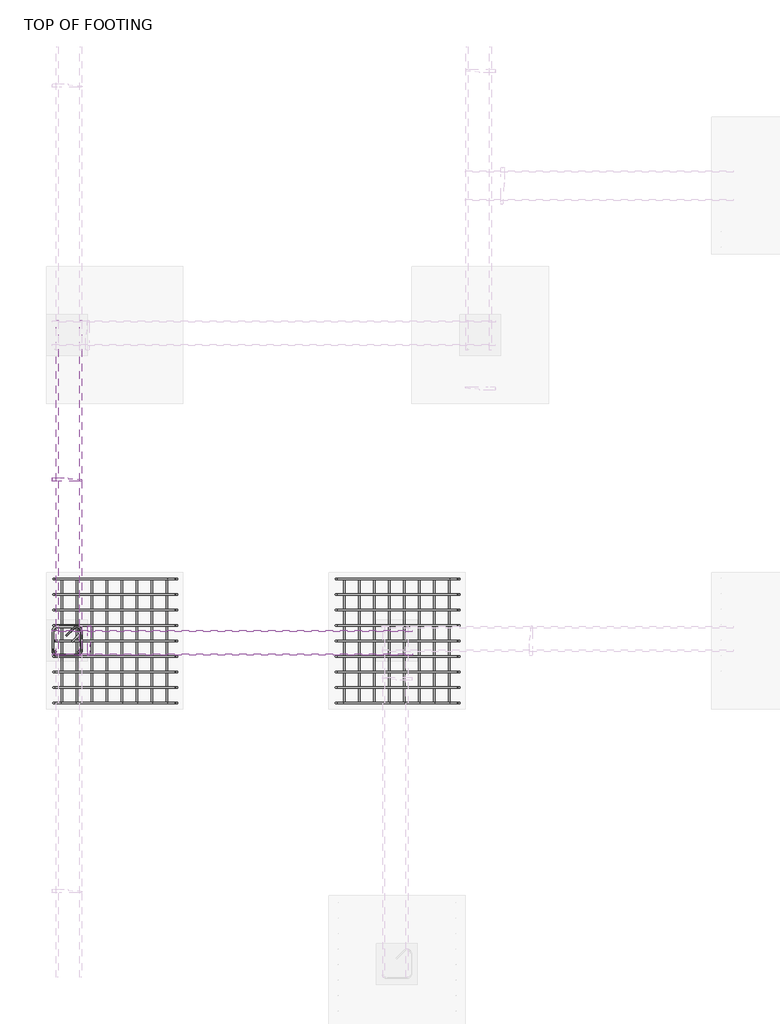
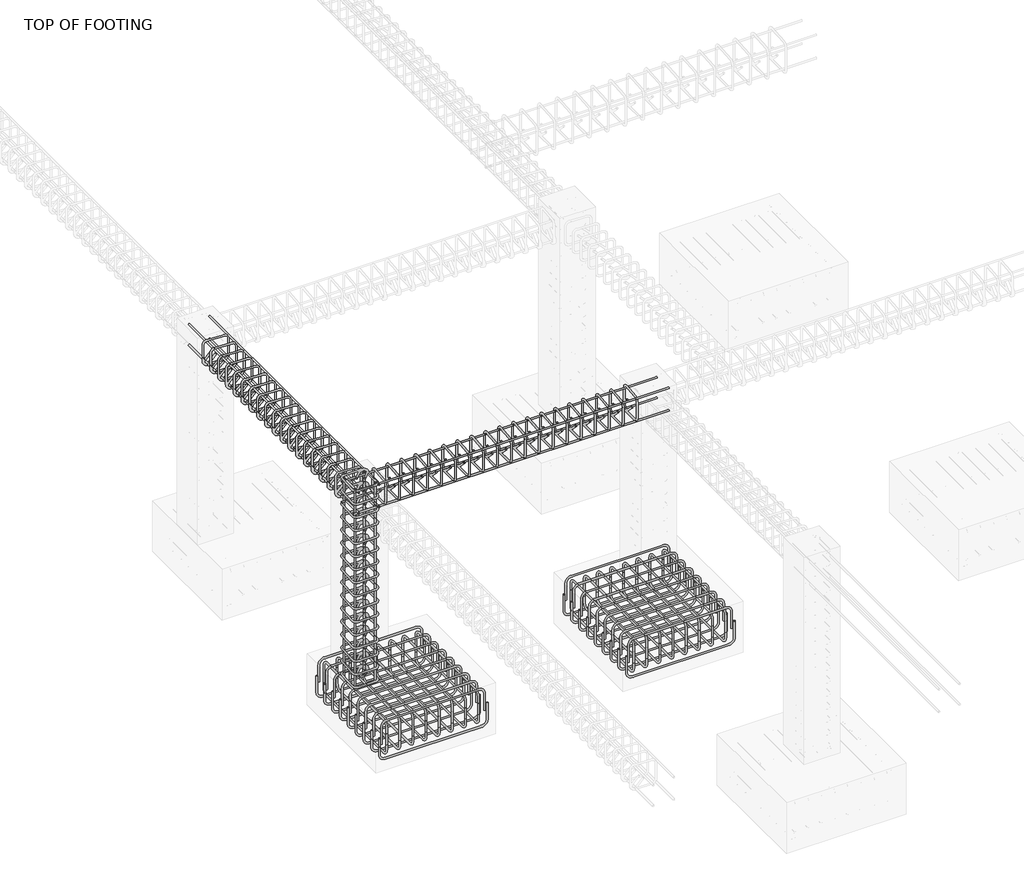
# One storey, part 4 of 10: 17 reinforcing bars.
"""IFC4 building model written with IfcOpenShell, lengths in millimetres."""

from ifc_helpers import new_model, si_unit, point, frame, origin, place, context, project, spatial, polyline, circle_curve, trimmed, segment, composite_curve, source, transform, mapped, element, save
from ifc_brep_helpers import swept_disk

model = new_model("IFC4")

# Units and contexts
model_context = context("Model", 3, world=origin())
ifc_project = project(units=[si_unit("LENGTHUNIT", "METRE", prefix="MILLI")], contexts=[model_context])

# Site, building, storey
site = spatial("IfcSite", under=ifc_project)
building = spatial("IfcBuilding", under=site)
storey = spatial("IfcBuildingStorey", under=building, Name="TOP OF FOOTING", Elevation=-1828.8)

# Reinforcing bars
placement = place(None, origin())
reinforcing_bar_shape = source(origin(), model_context, "Body", "SolidModel", [
    swept_disk(composite_curve([segment(polyline([(-9737.3957678, 12780.6767485, -2013.6880036), (-9737.3957678, 12780.6767485, -2160.9880036)]), True, "CONTINUOUS"), segment(trimmed(circle_curve(frame((-9783.7457678, 12780.6767485, -2160.9880036), z_axis=(0.0, 1.0, 0.0), x_axis=(46.349999999998545, 0.0, 0.0)), 46.35), [point((-9737.3957678, 12780.6767485, -2160.9880036))], [point((-9783.7457678, 12780.6767485, -2207.3380036))], True, "CARTESIAN"), True, "CONTINUOUS"), segment(polyline([(-9783.7457678, 12780.6767485, -2207.3380036), (-10591.4530437, 12780.6767485, -2207.3380036)]), True, "CONTINUOUS"), segment(trimmed(circle_curve(frame((-10591.4530437, 12780.6767485, -2160.9880036), z_axis=(0.0, 1.0, 0.0), x_axis=(0.0, 0.0, -46.34999999999991)), 46.35), [point((-10591.4530437, 12780.6767485, -2207.3380036))], [point((-10637.8030437, 12780.6767485, -2160.9880036))], True, "CARTESIAN"), True, "CONTINUOUS"), segment(polyline([(-10637.8030437, 12780.6767485, -2160.9880036), (-10637.8030437, 12780.6767485, -2013.6880036)]), True, "CONTINUOUS")], self_intersect=False), 6.35),
])
element("IfcReinforcingBar", 1, at=placement, inside=storey, context=model_context, shape_type="MappedRepresentation", body=[
    mapped(reinforcing_bar_shape, transform((0.0, 0.0, 0.0), x_axis=(1.0, 0.0, 0.0), y_axis=(0.0, 1.0, 0.0), z_axis=(0.0, 0.0, 1.0))),
    mapped(reinforcing_bar_shape, transform((0.0, -113.4125, 0.0), x_axis=(1.0, 0.0, 0.0), y_axis=(0.0, 1.0, 0.0), z_axis=(0.0, 0.0, 1.0))),
    mapped(reinforcing_bar_shape, transform((0.0, -226.825, 0.0), x_axis=(1.0, 0.0, 0.0), y_axis=(0.0, 1.0, 0.0), z_axis=(0.0, 0.0, 1.0))),
    mapped(reinforcing_bar_shape, transform((0.0, -340.2375, 0.0), x_axis=(1.0, 0.0, 0.0), y_axis=(0.0, 1.0, 0.0), z_axis=(0.0, 0.0, 1.0))),
    mapped(reinforcing_bar_shape, transform((0.0, -453.65, 0.0), x_axis=(1.0, 0.0, 0.0), y_axis=(0.0, 1.0, 0.0), z_axis=(0.0, 0.0, 1.0))),
    mapped(reinforcing_bar_shape, transform((0.0, -567.0625, 0.0), x_axis=(1.0, 0.0, 0.0), y_axis=(0.0, 1.0, 0.0), z_axis=(0.0, 0.0, 1.0))),
    mapped(reinforcing_bar_shape, transform((0.0, -680.475, 0.0), x_axis=(1.0, 0.0, 0.0), y_axis=(0.0, 1.0, 0.0), z_axis=(0.0, 0.0, 1.0))),
    mapped(reinforcing_bar_shape, transform((0.0, -793.8875, 0.0), x_axis=(1.0, 0.0, 0.0), y_axis=(0.0, 1.0, 0.0), z_axis=(0.0, 0.0, 1.0))),
    mapped(reinforcing_bar_shape, transform((0.0, -907.3, 0.0), x_axis=(1.0, 0.0, 0.0), y_axis=(0.0, 1.0, 0.0), z_axis=(0.0, 0.0, 1.0))),
])
reinforcing_bar_2_shape = source(origin(), model_context, "Body", "SolidModel", [
    swept_disk(composite_curve([segment(polyline([(-10621.5548549, 12780.6767485, -2068.7560969), (-10621.5548549, 12780.6767485, -1921.4560969)]), True, "CONTINUOUS"), segment(trimmed(circle_curve(frame((-10575.2048549, 12780.6767485, -1921.4560969), z_axis=(0.0, 1.0, 0.0), x_axis=(-46.350000000000364, 0.0, 0.0)), 46.35), [point((-10621.5548549, 12780.6767485, -1921.4560969))], [point((-10575.2048549, 12780.6767485, -1875.1060969))], True, "CARTESIAN"), True, "CONTINUOUS"), segment(polyline([(-10575.2048549, 12780.6767485, -1875.1060969), (-9806.8133686, 12780.6767485, -1875.1060969)]), True, "CONTINUOUS"), segment(trimmed(circle_curve(frame((-9806.8133686, 12780.6767485, -1921.4560969), z_axis=(0.0, 1.0, 0.0), x_axis=(0.0, 0.0, 46.34999999999991)), 46.35), [point((-9806.8133686, 12780.6767485, -1875.1060969))], [point((-9760.4633686, 12780.6767485, -1921.4560969))], True, "CARTESIAN"), True, "CONTINUOUS"), segment(polyline([(-9760.4633686, 12780.6767485, -1921.4560969), (-9760.4633686, 12780.6767485, -2068.7560969)]), True, "CONTINUOUS")], self_intersect=False), 6.35),
])
element("IfcReinforcingBar", 2, at=placement, inside=storey, context=model_context, shape_type="MappedRepresentation", body=[
    mapped(reinforcing_bar_2_shape, transform((0.0, 0.0, 0.0), x_axis=(1.0, 0.0, 0.0), y_axis=(0.0, 1.0, 0.0), z_axis=(0.0, 0.0, 1.0))),
    mapped(reinforcing_bar_2_shape, transform((0.0, -113.4125, 0.0), x_axis=(1.0, 0.0, 0.0), y_axis=(0.0, 1.0, 0.0), z_axis=(0.0, 0.0, 1.0))),
    mapped(reinforcing_bar_2_shape, transform((0.0, -226.825, 0.0), x_axis=(1.0, 0.0, 0.0), y_axis=(0.0, 1.0, 0.0), z_axis=(0.0, 0.0, 1.0))),
    mapped(reinforcing_bar_2_shape, transform((0.0, -340.2375, 0.0), x_axis=(1.0, 0.0, 0.0), y_axis=(0.0, 1.0, 0.0), z_axis=(0.0, 0.0, 1.0))),
    mapped(reinforcing_bar_2_shape, transform((0.0, -453.65, 0.0), x_axis=(1.0, 0.0, 0.0), y_axis=(0.0, 1.0, 0.0), z_axis=(0.0, 0.0, 1.0))),
    mapped(reinforcing_bar_2_shape, transform((0.0, -567.0625, 0.0), x_axis=(1.0, 0.0, 0.0), y_axis=(0.0, 1.0, 0.0), z_axis=(0.0, 0.0, 1.0))),
    mapped(reinforcing_bar_2_shape, transform((0.0, -680.475, 0.0), x_axis=(1.0, 0.0, 0.0), y_axis=(0.0, 1.0, 0.0), z_axis=(0.0, 0.0, 1.0))),
    mapped(reinforcing_bar_2_shape, transform((0.0, -793.8875, 0.0), x_axis=(1.0, 0.0, 0.0), y_axis=(0.0, 1.0, 0.0), z_axis=(0.0, 0.0, 1.0))),
    mapped(reinforcing_bar_2_shape, transform((0.0, -907.3, 0.0), x_axis=(1.0, 0.0, 0.0), y_axis=(0.0, 1.0, 0.0), z_axis=(0.0, 0.0, 1.0))),
])
reinforcing_bar_3_shape = source(origin(), model_context, "Body", "SolidModel", [
    swept_disk(composite_curve([segment(polyline([(-9809.6682872, 12780.6767485, -2087.4821199), (-9809.6682872, 12780.6767485, -1940.1821199)]), True, "CONTINUOUS"), segment(trimmed(circle_curve(frame((-9809.6682872, 12734.3267485, -1940.1821199), z_axis=(1.0, 0.0, 0.0), x_axis=(0.0, 46.350000000000364, 0.0)), 46.35), [point((-9809.6682872, 12780.6767485, -1940.1821199))], [point((-9809.6682872, 12734.3267485, -1893.8321199))], True, "CARTESIAN"), True, "CONTINUOUS"), segment(polyline([(-9809.6682872, 12734.3267485, -1893.8321199), (-9809.6682872, 11919.7267485, -1893.8321199)]), True, "CONTINUOUS"), segment(trimmed(circle_curve(frame((-9809.6682872, 11919.7267485, -1940.1821199), z_axis=(1.0, 0.0, 0.0), x_axis=(0.0, 0.0, 46.350000000000136)), 46.35), [point((-9809.6682872, 11919.7267485, -1893.8321199))], [point((-9809.6682872, 11873.3767485, -1940.1821199))], True, "CARTESIAN"), True, "CONTINUOUS"), segment(polyline([(-9809.6682872, 11873.3767485, -1940.1821199), (-9809.6682872, 11873.3767485, -2087.4821199)]), True, "CONTINUOUS")], self_intersect=False), 6.35),
])
element("IfcReinforcingBar", 3, at=placement, inside=storey, context=model_context, shape_type="MappedRepresentation", body=[
    mapped(reinforcing_bar_3_shape, transform((0.0, 0.0, 0.0), x_axis=(1.0, 0.0, 0.0), y_axis=(0.0, 1.0, 0.0), z_axis=(0.0, 0.0, 1.0))),
    mapped(reinforcing_bar_3_shape, transform((-109.824938, 0.0, 0.0), x_axis=(1.0, 0.0, 0.0), y_axis=(0.0, 1.0, 0.0), z_axis=(0.0, 0.0, 1.0))),
    mapped(reinforcing_bar_3_shape, transform((-219.649876, 0.0, 0.0), x_axis=(1.0, 0.0, 0.0), y_axis=(0.0, 1.0, 0.0), z_axis=(0.0, 0.0, 1.0))),
    mapped(reinforcing_bar_3_shape, transform((-329.474814, 0.0, 0.0), x_axis=(1.0, 0.0, 0.0), y_axis=(0.0, 1.0, 0.0), z_axis=(0.0, 0.0, 1.0))),
    mapped(reinforcing_bar_3_shape, transform((-439.299752, 0.0, 0.0), x_axis=(1.0, 0.0, 0.0), y_axis=(0.0, 1.0, 0.0), z_axis=(0.0, 0.0, 1.0))),
    mapped(reinforcing_bar_3_shape, transform((-549.12469, 0.0, 0.0), x_axis=(1.0, 0.0, 0.0), y_axis=(0.0, 1.0, 0.0), z_axis=(0.0, 0.0, 1.0))),
    mapped(reinforcing_bar_3_shape, transform((-658.949628, 0.0, 0.0), x_axis=(1.0, 0.0, 0.0), y_axis=(0.0, 1.0, 0.0), z_axis=(0.0, 0.0, 1.0))),
    mapped(reinforcing_bar_3_shape, transform((-768.774566, 0.0, 0.0), x_axis=(1.0, 0.0, 0.0), y_axis=(0.0, 1.0, 0.0), z_axis=(0.0, 0.0, 1.0))),
])
reinforcing_bar_4_shape = source(origin(), model_context, "Body", "SolidModel", [
    swept_disk(composite_curve([segment(polyline([(-10578.4428532, 12780.6767485, -1990.1985611), (-10578.4428532, 12780.6767485, -2137.4985611)]), True, "CONTINUOUS"), segment(trimmed(circle_curve(frame((-10578.4428532, 12734.3267485, -2137.4985611), z_axis=(-1.0, 0.0, 0.0), x_axis=(0.0, 46.350000000000364, 0.0)), 46.35), [point((-10578.4428532, 12780.6767485, -2137.4985611))], [point((-10578.4428532, 12734.3267485, -2183.8485611))], True, "CARTESIAN"), True, "CONTINUOUS"), segment(polyline([(-10578.4428532, 12734.3267485, -2183.8485611), (-10578.4428532, 11919.7267485, -2183.8485611)]), True, "CONTINUOUS"), segment(trimmed(circle_curve(frame((-10578.4428532, 11919.7267485, -2137.4985611), z_axis=(-1.0, 0.0, 0.0), x_axis=(0.0, 0.0, -46.34999999999991)), 46.35), [point((-10578.4428532, 11919.7267485, -2183.8485611))], [point((-10578.4428532, 11873.3767485, -2137.4985611))], True, "CARTESIAN"), True, "CONTINUOUS"), segment(polyline([(-10578.4428532, 11873.3767485, -2137.4985611), (-10578.4428532, 11873.3767485, -1990.1985611)]), True, "CONTINUOUS")], self_intersect=False), 6.35),
])
element("IfcReinforcingBar", 4, at=placement, inside=storey, context=model_context, shape_type="MappedRepresentation", body=[
    mapped(reinforcing_bar_4_shape, transform((0.0, 0.0, 0.0), x_axis=(1.0, 0.0, 0.0), y_axis=(0.0, 1.0, 0.0), z_axis=(0.0, 0.0, 1.0))),
    mapped(reinforcing_bar_4_shape, transform((109.824938, 0.0, 0.0), x_axis=(1.0, 0.0, 0.0), y_axis=(0.0, 1.0, 0.0), z_axis=(0.0, 0.0, 1.0))),
    mapped(reinforcing_bar_4_shape, transform((219.649876, 0.0, 0.0), x_axis=(1.0, 0.0, 0.0), y_axis=(0.0, 1.0, 0.0), z_axis=(0.0, 0.0, 1.0))),
    mapped(reinforcing_bar_4_shape, transform((329.474814, 0.0, 0.0), x_axis=(1.0, 0.0, 0.0), y_axis=(0.0, 1.0, 0.0), z_axis=(0.0, 0.0, 1.0))),
    mapped(reinforcing_bar_4_shape, transform((439.299752, 0.0, 0.0), x_axis=(1.0, 0.0, 0.0), y_axis=(0.0, 1.0, 0.0), z_axis=(0.0, 0.0, 1.0))),
    mapped(reinforcing_bar_4_shape, transform((549.12469, 0.0, 0.0), x_axis=(1.0, 0.0, 0.0), y_axis=(0.0, 1.0, 0.0), z_axis=(0.0, 0.0, 1.0))),
    mapped(reinforcing_bar_4_shape, transform((658.949628, 0.0, 0.0), x_axis=(1.0, 0.0, 0.0), y_axis=(0.0, 1.0, 0.0), z_axis=(0.0, 0.0, 1.0))),
    mapped(reinforcing_bar_4_shape, transform((768.774566, 0.0, 0.0), x_axis=(1.0, 0.0, 0.0), y_axis=(0.0, 1.0, 0.0), z_axis=(0.0, 0.0, 1.0))),
])
reinforcing_bar_5_shape = source(origin(), model_context, "Body", "SolidModel", [
    swept_disk(composite_curve([segment(polyline([(-7671.9957678, 12780.6767485, -2013.6880036), (-7671.9957678, 12780.6767485, -2160.9880036)]), True, "CONTINUOUS"), segment(trimmed(circle_curve(frame((-7718.3457678, 12780.6767485, -2160.9880036), z_axis=(0.0, 1.0, 0.0), x_axis=(46.350000000000364, 0.0, 0.0)), 46.35), [point((-7671.9957678, 12780.6767485, -2160.9880036))], [point((-7718.3457678, 12780.6767485, -2207.3380036))], True, "CARTESIAN"), True, "CONTINUOUS"), segment(polyline([(-7718.3457678, 12780.6767485, -2207.3380036), (-8526.0530437, 12780.6767485, -2207.3380036)]), True, "CONTINUOUS"), segment(trimmed(circle_curve(frame((-8526.0530437, 12780.6767485, -2160.9880036), z_axis=(0.0, 1.0, 0.0), x_axis=(0.0, 0.0, -46.34999999999991)), 46.35), [point((-8526.0530437, 12780.6767485, -2207.3380036))], [point((-8572.4030437, 12780.6767485, -2160.9880036))], True, "CARTESIAN"), True, "CONTINUOUS"), segment(polyline([(-8572.4030437, 12780.6767485, -2160.9880036), (-8572.4030437, 12780.6767485, -2013.6880036)]), True, "CONTINUOUS")], self_intersect=False), 6.35),
])
element("IfcReinforcingBar", 5, at=placement, inside=storey, context=model_context, shape_type="MappedRepresentation", body=[
    mapped(reinforcing_bar_5_shape, transform((0.0, 0.0, 0.0), x_axis=(1.0, 0.0, 0.0), y_axis=(0.0, 1.0, 0.0), z_axis=(0.0, 0.0, 1.0))),
    mapped(reinforcing_bar_5_shape, transform((0.0, -113.4125, 0.0), x_axis=(1.0, 0.0, 0.0), y_axis=(0.0, 1.0, 0.0), z_axis=(0.0, 0.0, 1.0))),
    mapped(reinforcing_bar_5_shape, transform((0.0, -226.825, 0.0), x_axis=(1.0, 0.0, 0.0), y_axis=(0.0, 1.0, 0.0), z_axis=(0.0, 0.0, 1.0))),
    mapped(reinforcing_bar_5_shape, transform((0.0, -340.2375, 0.0), x_axis=(1.0, 0.0, 0.0), y_axis=(0.0, 1.0, 0.0), z_axis=(0.0, 0.0, 1.0))),
    mapped(reinforcing_bar_5_shape, transform((0.0, -453.65, 0.0), x_axis=(1.0, 0.0, 0.0), y_axis=(0.0, 1.0, 0.0), z_axis=(0.0, 0.0, 1.0))),
    mapped(reinforcing_bar_5_shape, transform((0.0, -567.0625, 0.0), x_axis=(1.0, 0.0, 0.0), y_axis=(0.0, 1.0, 0.0), z_axis=(0.0, 0.0, 1.0))),
    mapped(reinforcing_bar_5_shape, transform((0.0, -680.475, 0.0), x_axis=(1.0, 0.0, 0.0), y_axis=(0.0, 1.0, 0.0), z_axis=(0.0, 0.0, 1.0))),
    mapped(reinforcing_bar_5_shape, transform((0.0, -793.8875, 0.0), x_axis=(1.0, 0.0, 0.0), y_axis=(0.0, 1.0, 0.0), z_axis=(0.0, 0.0, 1.0))),
    mapped(reinforcing_bar_5_shape, transform((0.0, -907.3, 0.0), x_axis=(1.0, 0.0, 0.0), y_axis=(0.0, 1.0, 0.0), z_axis=(0.0, 0.0, 1.0))),
])
reinforcing_bar_6_shape = source(origin(), model_context, "Body", "SolidModel", [
    swept_disk(composite_curve([segment(polyline([(-8556.1548549, 12780.6767485, -2068.7560969), (-8556.1548549, 12780.6767485, -1921.4560969)]), True, "CONTINUOUS"), segment(trimmed(circle_curve(frame((-8509.8048549, 12780.6767485, -1921.4560969), z_axis=(0.0, 1.0, 0.0), x_axis=(-46.350000000000364, 0.0, 0.0)), 46.35), [point((-8556.1548549, 12780.6767485, -1921.4560969))], [point((-8509.8048549, 12780.6767485, -1875.1060969))], True, "CARTESIAN"), True, "CONTINUOUS"), segment(polyline([(-8509.8048549, 12780.6767485, -1875.1060969), (-7741.4133686, 12780.6767485, -1875.1060969)]), True, "CONTINUOUS"), segment(trimmed(circle_curve(frame((-7741.4133686, 12780.6767485, -1921.4560969), z_axis=(0.0, 1.0, 0.0), x_axis=(0.0, 0.0, 46.34999999999991)), 46.35), [point((-7741.4133686, 12780.6767485, -1875.1060969))], [point((-7695.0633686, 12780.6767485, -1921.4560969))], True, "CARTESIAN"), True, "CONTINUOUS"), segment(polyline([(-7695.0633686, 12780.6767485, -1921.4560969), (-7695.0633686, 12780.6767485, -2068.7560969)]), True, "CONTINUOUS")], self_intersect=False), 6.35),
])
element("IfcReinforcingBar", 6, at=placement, inside=storey, context=model_context, shape_type="MappedRepresentation", body=[
    mapped(reinforcing_bar_6_shape, transform((0.0, 0.0, 0.0), x_axis=(1.0, 0.0, 0.0), y_axis=(0.0, 1.0, 0.0), z_axis=(0.0, 0.0, 1.0))),
    mapped(reinforcing_bar_6_shape, transform((0.0, -113.4125, 0.0), x_axis=(1.0, 0.0, 0.0), y_axis=(0.0, 1.0, 0.0), z_axis=(0.0, 0.0, 1.0))),
    mapped(reinforcing_bar_6_shape, transform((0.0, -226.825, 0.0), x_axis=(1.0, 0.0, 0.0), y_axis=(0.0, 1.0, 0.0), z_axis=(0.0, 0.0, 1.0))),
    mapped(reinforcing_bar_6_shape, transform((0.0, -340.2375, 0.0), x_axis=(1.0, 0.0, 0.0), y_axis=(0.0, 1.0, 0.0), z_axis=(0.0, 0.0, 1.0))),
    mapped(reinforcing_bar_6_shape, transform((0.0, -453.65, 0.0), x_axis=(1.0, 0.0, 0.0), y_axis=(0.0, 1.0, 0.0), z_axis=(0.0, 0.0, 1.0))),
    mapped(reinforcing_bar_6_shape, transform((0.0, -567.0625, 0.0), x_axis=(1.0, 0.0, 0.0), y_axis=(0.0, 1.0, 0.0), z_axis=(0.0, 0.0, 1.0))),
    mapped(reinforcing_bar_6_shape, transform((0.0, -680.475, 0.0), x_axis=(1.0, 0.0, 0.0), y_axis=(0.0, 1.0, 0.0), z_axis=(0.0, 0.0, 1.0))),
    mapped(reinforcing_bar_6_shape, transform((0.0, -793.8875, 0.0), x_axis=(1.0, 0.0, 0.0), y_axis=(0.0, 1.0, 0.0), z_axis=(0.0, 0.0, 1.0))),
    mapped(reinforcing_bar_6_shape, transform((0.0, -907.3, 0.0), x_axis=(1.0, 0.0, 0.0), y_axis=(0.0, 1.0, 0.0), z_axis=(0.0, 0.0, 1.0))),
])
reinforcing_bar_7_shape = source(origin(), model_context, "Body", "SolidModel", [
    swept_disk(composite_curve([segment(polyline([(-7744.2682872, 12780.6767485, -2087.4821199), (-7744.2682872, 12780.6767485, -1940.1821199)]), True, "CONTINUOUS"), segment(trimmed(circle_curve(frame((-7744.2682872, 12734.3267485, -1940.1821199), z_axis=(1.0, 0.0, 0.0), x_axis=(0.0, 46.350000000000364, 0.0)), 46.35), [point((-7744.2682872, 12780.6767485, -1940.1821199))], [point((-7744.2682872, 12734.3267485, -1893.8321199))], True, "CARTESIAN"), True, "CONTINUOUS"), segment(polyline([(-7744.2682872, 12734.3267485, -1893.8321199), (-7744.2682872, 11919.7267485, -1893.8321199)]), True, "CONTINUOUS"), segment(trimmed(circle_curve(frame((-7744.2682872, 11919.7267485, -1940.1821199), z_axis=(1.0, 0.0, 0.0), x_axis=(0.0, 0.0, 46.350000000000136)), 46.35), [point((-7744.2682872, 11919.7267485, -1893.8321199))], [point((-7744.2682872, 11873.3767485, -1940.1821199))], True, "CARTESIAN"), True, "CONTINUOUS"), segment(polyline([(-7744.2682872, 11873.3767485, -1940.1821199), (-7744.2682872, 11873.3767485, -2087.4821199)]), True, "CONTINUOUS")], self_intersect=False), 6.35),
])
element("IfcReinforcingBar", 7, at=placement, inside=storey, context=model_context, shape_type="MappedRepresentation", body=[
    mapped(reinforcing_bar_7_shape, transform((0.0, 0.0, 0.0), x_axis=(1.0, 0.0, 0.0), y_axis=(0.0, 1.0, 0.0), z_axis=(0.0, 0.0, 1.0))),
    mapped(reinforcing_bar_7_shape, transform((-109.824938, 0.0, 0.0), x_axis=(1.0, 0.0, 0.0), y_axis=(0.0, 1.0, 0.0), z_axis=(0.0, 0.0, 1.0))),
    mapped(reinforcing_bar_7_shape, transform((-219.649876, 0.0, 0.0), x_axis=(1.0, 0.0, 0.0), y_axis=(0.0, 1.0, 0.0), z_axis=(0.0, 0.0, 1.0))),
    mapped(reinforcing_bar_7_shape, transform((-329.474814, 0.0, 0.0), x_axis=(1.0, 0.0, 0.0), y_axis=(0.0, 1.0, 0.0), z_axis=(0.0, 0.0, 1.0))),
    mapped(reinforcing_bar_7_shape, transform((-439.299752, 0.0, 0.0), x_axis=(1.0, 0.0, 0.0), y_axis=(0.0, 1.0, 0.0), z_axis=(0.0, 0.0, 1.0))),
    mapped(reinforcing_bar_7_shape, transform((-549.12469, 0.0, 0.0), x_axis=(1.0, 0.0, 0.0), y_axis=(0.0, 1.0, 0.0), z_axis=(0.0, 0.0, 1.0))),
    mapped(reinforcing_bar_7_shape, transform((-658.949628, 0.0, 0.0), x_axis=(1.0, 0.0, 0.0), y_axis=(0.0, 1.0, 0.0), z_axis=(0.0, 0.0, 1.0))),
    mapped(reinforcing_bar_7_shape, transform((-768.774566, 0.0, 0.0), x_axis=(1.0, 0.0, 0.0), y_axis=(0.0, 1.0, 0.0), z_axis=(0.0, 0.0, 1.0))),
])
reinforcing_bar_8_shape = source(origin(), model_context, "Body", "SolidModel", [
    swept_disk(composite_curve([segment(polyline([(-8513.0428532, 12780.6767485, -1990.1985611), (-8513.0428532, 12780.6767485, -2137.4985611)]), True, "CONTINUOUS"), segment(trimmed(circle_curve(frame((-8513.0428532, 12734.3267485, -2137.4985611), z_axis=(-1.0, 0.0, 0.0), x_axis=(0.0, 46.350000000000364, 0.0)), 46.35), [point((-8513.0428532, 12780.6767485, -2137.4985611))], [point((-8513.0428532, 12734.3267485, -2183.8485611))], True, "CARTESIAN"), True, "CONTINUOUS"), segment(polyline([(-8513.0428532, 12734.3267485, -2183.8485611), (-8513.0428532, 11919.7267485, -2183.8485611)]), True, "CONTINUOUS"), segment(trimmed(circle_curve(frame((-8513.0428532, 11919.7267485, -2137.4985611), z_axis=(-1.0, 0.0, 0.0), x_axis=(0.0, 0.0, -46.34999999999991)), 46.35), [point((-8513.0428532, 11919.7267485, -2183.8485611))], [point((-8513.0428532, 11873.3767485, -2137.4985611))], True, "CARTESIAN"), True, "CONTINUOUS"), segment(polyline([(-8513.0428532, 11873.3767485, -2137.4985611), (-8513.0428532, 11873.3767485, -1990.1985611)]), True, "CONTINUOUS")], self_intersect=False), 6.35),
])
element("IfcReinforcingBar", 8, at=placement, inside=storey, context=model_context, shape_type="MappedRepresentation", body=[
    mapped(reinforcing_bar_8_shape, transform((0.0, 0.0, 0.0), x_axis=(1.0, 0.0, 0.0), y_axis=(0.0, 1.0, 0.0), z_axis=(0.0, 0.0, 1.0))),
    mapped(reinforcing_bar_8_shape, transform((109.824938, 0.0, 0.0), x_axis=(1.0, 0.0, 0.0), y_axis=(0.0, 1.0, 0.0), z_axis=(0.0, 0.0, 1.0))),
    mapped(reinforcing_bar_8_shape, transform((219.649876, 0.0, 0.0), x_axis=(1.0, 0.0, 0.0), y_axis=(0.0, 1.0, 0.0), z_axis=(0.0, 0.0, 1.0))),
    mapped(reinforcing_bar_8_shape, transform((329.474814, 0.0, 0.0), x_axis=(1.0, 0.0, 0.0), y_axis=(0.0, 1.0, 0.0), z_axis=(0.0, 0.0, 1.0))),
    mapped(reinforcing_bar_8_shape, transform((439.299752, 0.0, 0.0), x_axis=(1.0, 0.0, 0.0), y_axis=(0.0, 1.0, 0.0), z_axis=(0.0, 0.0, 1.0))),
    mapped(reinforcing_bar_8_shape, transform((549.12469, 0.0, 0.0), x_axis=(1.0, 0.0, 0.0), y_axis=(0.0, 1.0, 0.0), z_axis=(0.0, 0.0, 1.0))),
    mapped(reinforcing_bar_8_shape, transform((658.949628, 0.0, 0.0), x_axis=(1.0, 0.0, 0.0), y_axis=(0.0, 1.0, 0.0), z_axis=(0.0, 0.0, 1.0))),
    mapped(reinforcing_bar_8_shape, transform((768.774566, 0.0, 0.0), x_axis=(1.0, 0.0, 0.0), y_axis=(0.0, 1.0, 0.0), z_axis=(0.0, 0.0, 1.0))),
])
reinforcing_bar_9_shape = source(origin(), model_context, "Body", "SolidModel", [
    swept_disk(composite_curve([segment(polyline([(-10546.6571284, 12365.7509831, -46.35), (-10490.9135654, 12421.4945461, -46.35)]), True, "CONTINUOUS"), segment(trimmed(circle_curve(frame((-10468.7457678, 12399.3267485, -46.35), z_axis=(0.0, 0.0, -1.0), x_axis=(-22.167797600000995, 22.167797600000995, 0.0)), 31.35), [point((-10490.9135654, 12421.4945461, -46.35))], [point((-10437.3957678, 12399.3267485, -46.35))], True, "CARTESIAN"), True, "CONTINUOUS"), segment(polyline([(-10437.3957678, 12399.3267485, -46.35), (-10437.3957678, 12254.7267485, -46.35)]), True, "CONTINUOUS"), segment(trimmed(circle_curve(frame((-10468.7457678, 12254.7267485, -46.35), z_axis=(0.0, 0.0, -1.0), x_axis=(31.349999999998545, 0.0, 0.0)), 31.35), [point((-10437.3957678, 12254.7267485, -46.35))], [point((-10468.7457678, 12223.3767485, -46.35))], True, "CARTESIAN"), True, "CONTINUOUS"), segment(polyline([(-10468.7457678, 12223.3767485, -46.35), (-10613.3457678, 12223.3767485, -46.35)]), True, "CONTINUOUS"), segment(trimmed(circle_curve(frame((-10613.3457678, 12254.6680812, -44.4329719), z_axis=(0.0, 0.06114922175001322, -0.9981286353368326), x_axis=(0.0, -31.291332699998748, -1.9170281000000031)), 31.35), [point((-10613.3457678, 12223.3767485, -46.35))], [point((-10644.6957678, 12254.6680812, -44.4329719))], True, "CARTESIAN"), True, "CONTINUOUS"), segment(polyline([(-10644.6957678, 12254.6680812, -44.4329719), (-10644.6957678, 12399.3854158, -35.5670281)]), True, "CONTINUOUS"), segment(trimmed(circle_curve(frame((-10613.3457678, 12399.3854158, -35.5670281), z_axis=(0.0, 0.06114922175001322, -0.9981286353368326), x_axis=(-31.350000000000364, 0.0, 0.0)), 31.35), [point((-10644.6957678, 12399.3854158, -35.5670281))], [point((-10613.3457678, 12430.6767485, -33.65))], True, "CARTESIAN"), True, "CONTINUOUS"), segment(polyline([(-10613.3457678, 12430.6767485, -33.65), (-10468.7457678, 12430.6767485, -33.65)]), True, "CONTINUOUS"), segment(trimmed(circle_curve(frame((-10468.7457678, 12399.3267485, -33.65), z_axis=(0.0, 0.0, -1.0), x_axis=(0.0, 31.350000000000364, 0.0)), 31.35), [point((-10468.7457678, 12430.6767485, -33.65))], [point((-10446.5779702, 12377.1589509, -33.65))], True, "CARTESIAN"), True, "CONTINUOUS"), segment(polyline([(-10446.5779702, 12377.1589509, -33.65), (-10502.3215332, 12321.4153879, -33.65)]), True, "CONTINUOUS")], self_intersect=False), 6.35),
])
element("IfcReinforcingBar", 9, at=placement, inside=storey, context=model_context, shape_type="MappedRepresentation", body=[
    mapped(reinforcing_bar_9_shape, transform((0.0, 0.0, 0.0), x_axis=(1.0, 0.0, 0.0), y_axis=(0.0, 1.0, 0.0), z_axis=(0.0, 0.0, 1.0))),
    mapped(reinforcing_bar_9_shape, transform((0.0, 0.0, -115.74), x_axis=(1.0, 0.0, 0.0), y_axis=(0.0, 1.0, 0.0), z_axis=(0.0, 0.0, 1.0))),
    mapped(reinforcing_bar_9_shape, transform((0.0, 0.0, -231.48), x_axis=(1.0, 0.0, 0.0), y_axis=(0.0, 1.0, 0.0), z_axis=(0.0, 0.0, 1.0))),
    mapped(reinforcing_bar_9_shape, transform((0.0, 0.0, -347.22), x_axis=(1.0, 0.0, 0.0), y_axis=(0.0, 1.0, 0.0), z_axis=(0.0, 0.0, 1.0))),
    mapped(reinforcing_bar_9_shape, transform((0.0, 0.0, -462.96), x_axis=(1.0, 0.0, 0.0), y_axis=(0.0, 1.0, 0.0), z_axis=(0.0, 0.0, 1.0))),
    mapped(reinforcing_bar_9_shape, transform((0.0, 0.0, -578.7), x_axis=(1.0, 0.0, 0.0), y_axis=(0.0, 1.0, 0.0), z_axis=(0.0, 0.0, 1.0))),
    mapped(reinforcing_bar_9_shape, transform((0.0, 0.0, -694.44), x_axis=(1.0, 0.0, 0.0), y_axis=(0.0, 1.0, 0.0), z_axis=(0.0, 0.0, 1.0))),
    mapped(reinforcing_bar_9_shape, transform((0.0, 0.0, -810.18), x_axis=(1.0, 0.0, 0.0), y_axis=(0.0, 1.0, 0.0), z_axis=(0.0, 0.0, 1.0))),
    mapped(reinforcing_bar_9_shape, transform((0.0, 0.0, -925.92), x_axis=(1.0, 0.0, 0.0), y_axis=(0.0, 1.0, 0.0), z_axis=(0.0, 0.0, 1.0))),
    mapped(reinforcing_bar_9_shape, transform((0.0, 0.0, -1041.66), x_axis=(1.0, 0.0, 0.0), y_axis=(0.0, 1.0, 0.0), z_axis=(0.0, 0.0, 1.0))),
    mapped(reinforcing_bar_9_shape, transform((0.0, 0.0, -1157.4), x_axis=(1.0, 0.0, 0.0), y_axis=(0.0, 1.0, 0.0), z_axis=(0.0, 0.0, 1.0))),
    mapped(reinforcing_bar_9_shape, transform((0.0, 0.0, -1273.14), x_axis=(1.0, 0.0, 0.0), y_axis=(0.0, 1.0, 0.0), z_axis=(0.0, 0.0, 1.0))),
    mapped(reinforcing_bar_9_shape, transform((0.0, 0.0, -1388.88), x_axis=(1.0, 0.0, 0.0), y_axis=(0.0, 1.0, 0.0), z_axis=(0.0, 0.0, 1.0))),
    mapped(reinforcing_bar_9_shape, transform((0.0, 0.0, -1504.62), x_axis=(1.0, 0.0, 0.0), y_axis=(0.0, 1.0, 0.0), z_axis=(0.0, 0.0, 1.0))),
    mapped(reinforcing_bar_9_shape, transform((0.0, 0.0, -1620.36), x_axis=(1.0, 0.0, 0.0), y_axis=(0.0, 1.0, 0.0), z_axis=(0.0, 0.0, 1.0))),
    mapped(reinforcing_bar_9_shape, transform((0.0, 0.0, -1736.1), x_axis=(1.0, 0.0, 0.0), y_axis=(0.0, 1.0, 0.0), z_axis=(0.0, 0.0, 1.0))),
])
reinforcing_bar_10_shape = source(origin(), model_context, "Body", "SolidModel", [
    swept_disk(composite_curve([segment(polyline([(-10458.1163335, 12406.8267485, -1788.8), (-10458.1163335, 12406.8267485, -40.0)]), True, "CONTINUOUS")], self_intersect=False), 6.35),
])
element("IfcReinforcingBar", 10, at=placement, inside=storey, context=model_context, shape_type="MappedRepresentation", body=[
    mapped(reinforcing_bar_10_shape, transform((0.0, 0.0, 0.0), x_axis=(1.0, 0.0, 0.0), y_axis=(0.0, 1.0, 0.0), z_axis=(0.0, 0.0, 1.0))),
    mapped(reinforcing_bar_10_shape, transform((-168.8572682, 0.0, 0.0), x_axis=(1.0, 0.0, 0.0), y_axis=(0.0, 1.0, 0.0), z_axis=(0.0, 0.0, 1.0))),
])
reinforcing_bar_11_shape = source(origin(), model_context, "Body", "SolidModel", [
    swept_disk(composite_curve([segment(polyline([(-10458.1163335, 12247.2267485, -1788.8), (-10458.1163335, 12247.2267485, -40.0)]), True, "CONTINUOUS")], self_intersect=False), 6.35),
])
element("IfcReinforcingBar", 11, at=placement, inside=storey, context=model_context, shape_type="MappedRepresentation", body=[
    mapped(reinforcing_bar_11_shape, transform((0.0, 0.0, 0.0), x_axis=(1.0, 0.0, 0.0), y_axis=(0.0, 1.0, 0.0), z_axis=(0.0, 0.0, 1.0))),
    mapped(reinforcing_bar_11_shape, transform((-168.8572682, 0.0, 0.0), x_axis=(1.0, 0.0, 0.0), y_axis=(0.0, 1.0, 0.0), z_axis=(0.0, 0.0, 1.0))),
])
reinforcing_bar_12_shape = source(origin(), model_context, "Body", "SolidModel", [
    swept_disk(composite_curve([segment(polyline([(-10579.7700025, 14405.8767485, -144.3886395), (-10635.5135654, 14405.8767485, -200.1322024)]), True, "CONTINUOUS"), segment(trimmed(circle_curve(frame((-10613.3457678, 14405.8767485, -222.3), z_axis=(0.0, -1.0, 0.0), x_axis=(-22.167797600000995, 0.0, 22.1677976)), 31.35), [point((-10635.5135654, 14405.8767485, -200.1322024))], [point((-10613.3457678, 14405.8767485, -253.65))], True, "CARTESIAN"), True, "CONTINUOUS"), segment(polyline([(-10613.3457678, 14405.8767485, -253.65), (-10468.7457678, 14405.8767485, -253.65)]), True, "CONTINUOUS"), segment(trimmed(circle_curve(frame((-10468.7457678, 14405.8767485, -222.3), z_axis=(0.0, -1.0, 0.0), x_axis=(0.0, 0.0, -31.349999999999994)), 31.35), [point((-10468.7457678, 14405.8767485, -253.65))], [point((-10437.3957678, 14405.8767485, -222.3))], True, "CARTESIAN"), True, "CONTINUOUS"), segment(polyline([(-10437.3957678, 14405.8767485, -222.3), (-10437.3957678, 14405.8767485, -77.7)]), True, "CONTINUOUS"), segment(trimmed(circle_curve(frame((-10468.6871006, 14407.7937766, -77.7), z_axis=(-0.06114922175001155, -0.9981286353368327, 0.0), x_axis=(31.29133279999951, -1.917028099998788, 0.0)), 31.35), [point((-10437.3957678, 14405.8767485, -77.7))], [point((-10468.6871006, 14407.7937766, -46.35))], True, "CARTESIAN"), True, "CONTINUOUS"), segment(polyline([(-10468.6871006, 14407.7937766, -46.35), (-10613.4044351, 14416.6597204, -46.35)]), True, "CONTINUOUS"), segment(trimmed(circle_curve(frame((-10613.4044351, 14416.6597204, -77.7), z_axis=(-0.06114922175001155, -0.9981286353368327, 0.0), x_axis=(0.0, 0.0, 31.35)), 31.35), [point((-10613.4044351, 14416.6597204, -46.35))], [point((-10644.6957678, 14418.5767485, -77.7))], True, "CARTESIAN"), True, "CONTINUOUS"), segment(polyline([(-10644.6957678, 14418.5767485, -77.7), (-10644.6957678, 14418.5767485, -222.3)]), True, "CONTINUOUS"), segment(trimmed(circle_curve(frame((-10613.3457678, 14418.5767485, -222.3), z_axis=(0.0, -1.0, 0.0), x_axis=(-31.350000000000364, 0.0, 0.0)), 31.35), [point((-10644.6957678, 14418.5767485, -222.3))], [point((-10591.1779702, 14418.5767485, -244.4677976))], True, "CARTESIAN"), True, "CONTINUOUS"), segment(polyline([(-10591.1779702, 14418.5767485, -244.4677976), (-10535.4344073, 14418.5767485, -188.7242346)]), True, "CONTINUOUS")], self_intersect=False), 6.35),
])
element("IfcReinforcingBar", 12, at=placement, inside=storey, context=model_context, shape_type="MappedRepresentation", body=[
    mapped(reinforcing_bar_12_shape, transform((0.0, 0.0, 0.0), x_axis=(1.0, 0.0, 0.0), y_axis=(0.0, 1.0, 0.0), z_axis=(0.0, 0.0, 1.0))),
    mapped(reinforcing_bar_12_shape, transform((0.0, -113.0882353, 0.0), x_axis=(1.0, 0.0, 0.0), y_axis=(0.0, 1.0, 0.0), z_axis=(0.0, 0.0, 1.0))),
    mapped(reinforcing_bar_12_shape, transform((0.0, -226.1764706, 0.0), x_axis=(1.0, 0.0, 0.0), y_axis=(0.0, 1.0, 0.0), z_axis=(0.0, 0.0, 1.0))),
    mapped(reinforcing_bar_12_shape, transform((0.0, -339.2647059, 0.0), x_axis=(1.0, 0.0, 0.0), y_axis=(0.0, 1.0, 0.0), z_axis=(0.0, 0.0, 1.0))),
    mapped(reinforcing_bar_12_shape, transform((0.0, -452.3529412, 0.0), x_axis=(1.0, 0.0, 0.0), y_axis=(0.0, 1.0, 0.0), z_axis=(0.0, 0.0, 1.0))),
    mapped(reinforcing_bar_12_shape, transform((0.0, -565.4411765, 0.0), x_axis=(1.0, 0.0, 0.0), y_axis=(0.0, 1.0, 0.0), z_axis=(0.0, 0.0, 1.0))),
    mapped(reinforcing_bar_12_shape, transform((0.0, -678.5294118, 0.0), x_axis=(1.0, 0.0, 0.0), y_axis=(0.0, 1.0, 0.0), z_axis=(0.0, 0.0, 1.0))),
    mapped(reinforcing_bar_12_shape, transform((0.0, -791.6176471, 0.0), x_axis=(1.0, 0.0, 0.0), y_axis=(0.0, 1.0, 0.0), z_axis=(0.0, 0.0, 1.0))),
    mapped(reinforcing_bar_12_shape, transform((0.0, -904.7058824, 0.0), x_axis=(1.0, 0.0, 0.0), y_axis=(0.0, 1.0, 0.0), z_axis=(0.0, 0.0, 1.0))),
    mapped(reinforcing_bar_12_shape, transform((0.0, -1017.7941176, 0.0), x_axis=(1.0, 0.0, 0.0), y_axis=(0.0, 1.0, 0.0), z_axis=(0.0, 0.0, 1.0))),
    mapped(reinforcing_bar_12_shape, transform((0.0, -1130.8823529, 0.0), x_axis=(1.0, 0.0, 0.0), y_axis=(0.0, 1.0, 0.0), z_axis=(0.0, 0.0, 1.0))),
    mapped(reinforcing_bar_12_shape, transform((0.0, -1243.9705882, 0.0), x_axis=(1.0, 0.0, 0.0), y_axis=(0.0, 1.0, 0.0), z_axis=(0.0, 0.0, 1.0))),
    mapped(reinforcing_bar_12_shape, transform((0.0, -1357.0588235, 0.0), x_axis=(1.0, 0.0, 0.0), y_axis=(0.0, 1.0, 0.0), z_axis=(0.0, 0.0, 1.0))),
    mapped(reinforcing_bar_12_shape, transform((0.0, -1470.1470588, 0.0), x_axis=(1.0, 0.0, 0.0), y_axis=(0.0, 1.0, 0.0), z_axis=(0.0, 0.0, 1.0))),
    mapped(reinforcing_bar_12_shape, transform((0.0, -1583.2352941, 0.0), x_axis=(1.0, 0.0, 0.0), y_axis=(0.0, 1.0, 0.0), z_axis=(0.0, 0.0, 1.0))),
    mapped(reinforcing_bar_12_shape, transform((0.0, -1696.3235294, 0.0), x_axis=(1.0, 0.0, 0.0), y_axis=(0.0, 1.0, 0.0), z_axis=(0.0, 0.0, 1.0))),
    mapped(reinforcing_bar_12_shape, transform((0.0, -1809.4117647, 0.0), x_axis=(1.0, 0.0, 0.0), y_axis=(0.0, 1.0, 0.0), z_axis=(0.0, 0.0, 1.0))),
    mapped(reinforcing_bar_12_shape, transform((0.0, -1922.5, 0.0), x_axis=(1.0, 0.0, 0.0), y_axis=(0.0, 1.0, 0.0), z_axis=(0.0, 0.0, 1.0))),
])
reinforcing_bar_13_shape = source(origin(), model_context, "Body", "SolidModel", [
    swept_disk(composite_curve([segment(polyline([(-10613.3457678, 14672.2267485, -240.95), (-10613.3457678, 12217.0267485, -240.95)]), True, "CONTINUOUS")], self_intersect=False), 6.35),
])
element("IfcReinforcingBar", 13, at=placement, inside=storey, context=model_context, shape_type="MappedRepresentation", body=[
    mapped(reinforcing_bar_13_shape, transform((0.0, 0.0, 0.0), x_axis=(1.0, 0.0, 0.0), y_axis=(0.0, 1.0, 0.0), z_axis=(0.0, 0.0, 1.0))),
    mapped(reinforcing_bar_13_shape, transform((0.0, 0.0, 181.9), x_axis=(1.0, 0.0, 0.0), y_axis=(0.0, 1.0, 0.0), z_axis=(0.0, 0.0, 1.0))),
])
reinforcing_bar_14_shape = source(origin(), model_context, "Body", "SolidModel", [
    swept_disk(composite_curve([segment(polyline([(-10441.7457678, 14672.2267485, -245.5918309), (-10441.7457678, 12217.0267485, -245.5918309)]), True, "CONTINUOUS")], self_intersect=False), 6.35),
])
element("IfcReinforcingBar", 14, at=placement, inside=storey, context=model_context, shape_type="MappedRepresentation", body=[
    mapped(reinforcing_bar_14_shape, transform((0.0, 0.0, 0.0), x_axis=(1.0, 0.0, 0.0), y_axis=(0.0, 1.0, 0.0), z_axis=(0.0, 0.0, 1.0))),
    mapped(reinforcing_bar_14_shape, transform((0.0, 0.0, 197.4676357), x_axis=(1.0, 0.0, 0.0), y_axis=(0.0, 1.0, 0.0), z_axis=(0.0, 0.0, 1.0))),
])
reinforcing_bar_15_shape = source(origin(), model_context, "Body", "SolidModel", [
    swept_disk(composite_curve([segment(polyline([(-8281.9957678, 12365.7509831, -144.3886395), (-8281.9957678, 12421.4945461, -200.1322024)]), True, "CONTINUOUS"), segment(trimmed(circle_curve(frame((-8281.9957678, 12399.3267485, -222.3), z_axis=(-1.0, 0.0, 0.0), x_axis=(0.0, 22.167797600000995, 22.1677976)), 31.35), [point((-8281.9957678, 12421.4945461, -200.1322024))], [point((-8281.9957678, 12399.3267485, -253.65))], True, "CARTESIAN"), True, "CONTINUOUS"), segment(polyline([(-8281.9957678, 12399.3267485, -253.65), (-8281.9957678, 12254.7267485, -253.65)]), True, "CONTINUOUS"), segment(trimmed(circle_curve(frame((-8281.9957678, 12254.7267485, -222.3), z_axis=(-1.0, 0.0, 0.0), x_axis=(0.0, 0.0, -31.349999999999994)), 31.35), [point((-8281.9957678, 12254.7267485, -253.65))], [point((-8281.9957678, 12223.3767485, -222.3))], True, "CARTESIAN"), True, "CONTINUOUS"), segment(polyline([(-8281.9957678, 12223.3767485, -222.3), (-8281.9957678, 12223.3767485, -77.7)]), True, "CONTINUOUS"), segment(trimmed(circle_curve(frame((-8280.0787397, 12254.6680812, -77.7), z_axis=(-0.9981286353368326, 0.0611492217500135, 0.0), x_axis=(-1.917028099998788, -31.291332699998748, 0.0)), 31.35), [point((-8281.9957678, 12223.3767485, -77.7))], [point((-8280.0787397, 12254.6680812, -46.35))], True, "CARTESIAN"), True, "CONTINUOUS"), segment(polyline([(-8280.0787397, 12254.6680812, -46.35), (-8271.2127959, 12399.3854158, -46.35)]), True, "CONTINUOUS"), segment(trimmed(circle_curve(frame((-8271.2127959, 12399.3854158, -77.7), z_axis=(-0.9981286353368326, 0.0611492217500135, 0.0), x_axis=(0.0, 0.0, 31.35)), 31.35), [point((-8271.2127959, 12399.3854158, -46.35))], [point((-8269.2957678, 12430.6767485, -77.7))], True, "CARTESIAN"), True, "CONTINUOUS"), segment(polyline([(-8269.2957678, 12430.6767485, -77.7), (-8269.2957678, 12430.6767485, -222.3)]), True, "CONTINUOUS"), segment(trimmed(circle_curve(frame((-8269.2957678, 12399.3267485, -222.3), z_axis=(-1.0, 0.0, 0.0), x_axis=(0.0, 31.350000000000364, 0.0)), 31.35), [point((-8269.2957678, 12430.6767485, -222.3))], [point((-8269.2957678, 12377.1589509, -244.4677976))], True, "CARTESIAN"), True, "CONTINUOUS"), segment(polyline([(-8269.2957678, 12377.1589509, -244.4677976), (-8269.2957678, 12321.4153879, -188.7242346)]), True, "CONTINUOUS")], self_intersect=False), 6.35),
])
element("IfcReinforcingBar", 15, at=placement, inside=storey, context=model_context, shape_type="MappedRepresentation", body=[
    mapped(reinforcing_bar_15_shape, transform((0.0, 0.0, 0.0), x_axis=(1.0, 0.0, 0.0), y_axis=(0.0, 1.0, 0.0), z_axis=(0.0, 0.0, 1.0))),
    mapped(reinforcing_bar_15_shape, transform((-116.8166667, 0.0, 0.0), x_axis=(1.0, 0.0, 0.0), y_axis=(0.0, 1.0, 0.0), z_axis=(0.0, 0.0, 1.0))),
    mapped(reinforcing_bar_15_shape, transform((-233.6333333, 0.0, 0.0), x_axis=(1.0, 0.0, 0.0), y_axis=(0.0, 1.0, 0.0), z_axis=(0.0, 0.0, 1.0))),
    mapped(reinforcing_bar_15_shape, transform((-350.45, 0.0, 0.0), x_axis=(1.0, 0.0, 0.0), y_axis=(0.0, 1.0, 0.0), z_axis=(0.0, 0.0, 1.0))),
    mapped(reinforcing_bar_15_shape, transform((-467.2666667, 0.0, 0.0), x_axis=(1.0, 0.0, 0.0), y_axis=(0.0, 1.0, 0.0), z_axis=(0.0, 0.0, 1.0))),
    mapped(reinforcing_bar_15_shape, transform((-584.0833333, 0.0, 0.0), x_axis=(1.0, 0.0, 0.0), y_axis=(0.0, 1.0, 0.0), z_axis=(0.0, 0.0, 1.0))),
    mapped(reinforcing_bar_15_shape, transform((-700.9, 0.0, 0.0), x_axis=(1.0, 0.0, 0.0), y_axis=(0.0, 1.0, 0.0), z_axis=(0.0, 0.0, 1.0))),
    mapped(reinforcing_bar_15_shape, transform((-817.7166667, 0.0, 0.0), x_axis=(1.0, 0.0, 0.0), y_axis=(0.0, 1.0, 0.0), z_axis=(0.0, 0.0, 1.0))),
    mapped(reinforcing_bar_15_shape, transform((-934.5333333, 0.0, 0.0), x_axis=(1.0, 0.0, 0.0), y_axis=(0.0, 1.0, 0.0), z_axis=(0.0, 0.0, 1.0))),
    mapped(reinforcing_bar_15_shape, transform((-1051.35, 0.0, 0.0), x_axis=(1.0, 0.0, 0.0), y_axis=(0.0, 1.0, 0.0), z_axis=(0.0, 0.0, 1.0))),
    mapped(reinforcing_bar_15_shape, transform((-1168.1666667, 0.0, 0.0), x_axis=(1.0, 0.0, 0.0), y_axis=(0.0, 1.0, 0.0), z_axis=(0.0, 0.0, 1.0))),
    mapped(reinforcing_bar_15_shape, transform((-1284.9833333, 0.0, 0.0), x_axis=(1.0, 0.0, 0.0), y_axis=(0.0, 1.0, 0.0), z_axis=(0.0, 0.0, 1.0))),
    mapped(reinforcing_bar_15_shape, transform((-1401.8, 0.0, 0.0), x_axis=(1.0, 0.0, 0.0), y_axis=(0.0, 1.0, 0.0), z_axis=(0.0, 0.0, 1.0))),
    mapped(reinforcing_bar_15_shape, transform((-1518.6166667, 0.0, 0.0), x_axis=(1.0, 0.0, 0.0), y_axis=(0.0, 1.0, 0.0), z_axis=(0.0, 0.0, 1.0))),
    mapped(reinforcing_bar_15_shape, transform((-1635.4333333, 0.0, 0.0), x_axis=(1.0, 0.0, 0.0), y_axis=(0.0, 1.0, 0.0), z_axis=(0.0, 0.0, 1.0))),
    mapped(reinforcing_bar_15_shape, transform((-1752.25, 0.0, 0.0), x_axis=(1.0, 0.0, 0.0), y_axis=(0.0, 1.0, 0.0), z_axis=(0.0, 0.0, 1.0))),
    mapped(reinforcing_bar_15_shape, transform((-1869.0666667, 0.0, 0.0), x_axis=(1.0, 0.0, 0.0), y_axis=(0.0, 1.0, 0.0), z_axis=(0.0, 0.0, 1.0))),
    mapped(reinforcing_bar_15_shape, transform((-1985.8833333, 0.0, 0.0), x_axis=(1.0, 0.0, 0.0), y_axis=(0.0, 1.0, 0.0), z_axis=(0.0, 0.0, 1.0))),
    mapped(reinforcing_bar_15_shape, transform((-2102.7, 0.0, 0.0), x_axis=(1.0, 0.0, 0.0), y_axis=(0.0, 1.0, 0.0), z_axis=(0.0, 0.0, 1.0))),
])
reinforcing_bar_16_shape = source(origin(), model_context, "Body", "SolidModel", [
    swept_disk(composite_curve([segment(polyline([(-8015.6457678, 12399.3267485, -240.95), (-10651.0457678, 12399.3267485, -240.95)]), True, "CONTINUOUS")], self_intersect=False), 6.35),
])
element("IfcReinforcingBar", 16, at=placement, inside=storey, context=model_context, shape_type="MappedRepresentation", body=[
    mapped(reinforcing_bar_16_shape, transform((0.0, 0.0, 0.0), x_axis=(1.0, 0.0, 0.0), y_axis=(0.0, 1.0, 0.0), z_axis=(0.0, 0.0, 1.0))),
    mapped(reinforcing_bar_16_shape, transform((0.0, 0.0, 181.9), x_axis=(1.0, 0.0, 0.0), y_axis=(0.0, 1.0, 0.0), z_axis=(0.0, 0.0, 1.0))),
])
reinforcing_bar_17_shape = source(origin(), model_context, "Body", "SolidModel", [
    swept_disk(composite_curve([segment(polyline([(-8015.6457678, 12227.7267485, -245.5918309), (-10651.0457678, 12227.7267485, -245.5918309)]), True, "CONTINUOUS")], self_intersect=False), 6.35),
])
element("IfcReinforcingBar", 17, at=placement, inside=storey, context=model_context, shape_type="MappedRepresentation", body=[
    mapped(reinforcing_bar_17_shape, transform((0.0, 0.0, 0.0), x_axis=(1.0, 0.0, 0.0), y_axis=(0.0, 1.0, 0.0), z_axis=(0.0, 0.0, 1.0))),
    mapped(reinforcing_bar_17_shape, transform((0.0, 0.0, 197.4676357), x_axis=(1.0, 0.0, 0.0), y_axis=(0.0, 1.0, 0.0), z_axis=(0.0, 0.0, 1.0))),
])

save(model, "model.ifc")

# Revit data of these elements
# Elements 1, 2, 3, 4, 5, 6, 7, 8, 9, 10, 11, 12, 13, 14, 15, 16, 17 (IfcReinforcingBar)
#   Phase Created = New Construction
